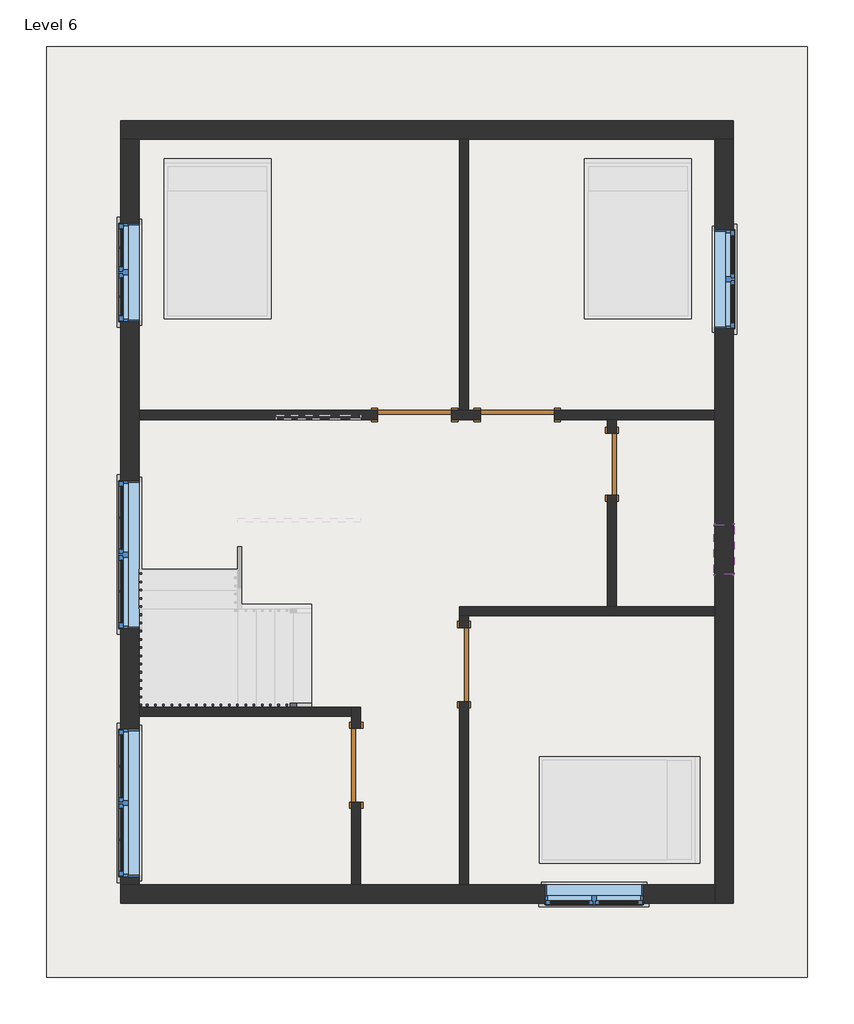
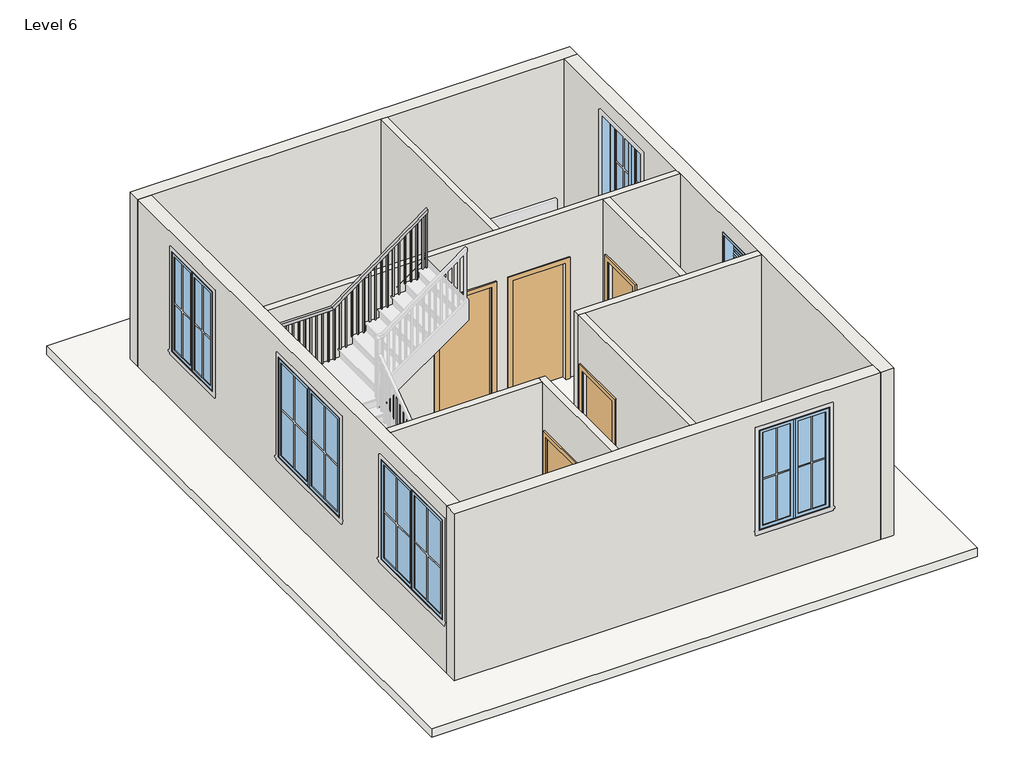
# One storey, part 1 of 2: 11 walls, 6 windows, 5 doors, 1 railing, 1 roof.
"""IFC4 building model written with IfcOpenShell, lengths in millimetres."""

from ifc_helpers import new_model, si_unit, frame, origin, place, context, project, spatial, polyline, outline, extrude, faceted_brep, transform, mapped, element, save
from components import door_f2b275c1, single_flush_door_3_e5f9f3c4, single_flush_door_3_305aa2a5, window_casement_double_win_4_6ca1769e, window_casement_double_win_6_ce442eab, window_f2d8fef0

model = new_model("IFC4")

# Units and contexts
model_context = context("Model", 3, world=origin())
ifc_project = project(units=[si_unit("LENGTHUNIT", "METRE", prefix="MILLI")], contexts=[model_context])

# Site, building, storey
site = spatial("IfcSite", under=ifc_project)
building = spatial("IfcBuilding", under=site)
storey = spatial("IfcBuildingStorey", under=building, Name="Level 6", Elevation=15849.6)

# Doors
placement = place(None, origin())
door_shape = door_f2b275c1(model_context)
element("IfcDoor", 1, ObjectType="Single-Flush : 2'6\"", at=placement, inside=storey, context=model_context, shape_type="MappedRepresentation", body=[
    mapped(door_shape, transform((1031.6394609, 262.5126239, 15849.6), x_axis=(0.0, 1.0, 0.0), y_axis=(-1.0, 0.0, 0.0), z_axis=(0.0, 0.0, 1.0))),
])
single_flush_door_3_shape = single_flush_door_3_e5f9f3c4(model_context)
element("IfcDoor", 2, ObjectType="Single-Flush : door 3'", at=placement, inside=storey, context=model_context, shape_type="MappedRepresentation", body=[
    mapped(single_flush_door_3_shape, transform((-1406.7605391, 872.1126239, 15849.6), x_axis=(1.0, 0.0, 0.0), y_axis=(0.0, 1.0, 0.0), z_axis=(0.0, 0.0, 1.0))),
])
element("IfcDoor", 3, ObjectType="Single-Flush : door 3'", at=placement, inside=storey, context=model_context, shape_type="MappedRepresentation", body=[
    mapped(single_flush_door_3_shape, transform((-2130.6605391, -3458.5873761, 15849.6), x_axis=(0.0, 1.0, 0.0), y_axis=(-1.0, 0.0, 0.0), z_axis=(0.0, 0.0, 1.0))),
])
single_flush_door_3_2_shape = single_flush_door_3_305aa2a5(model_context)
element("IfcDoor", 4, ObjectType="Single-Flush : door 3'", at=placement, inside=storey, context=model_context, shape_type="MappedRepresentation", body=[
    mapped(single_flush_door_3_2_shape, transform((-136.7605391, 872.1126239, 15849.6), x_axis=(-1.0, 0.0, 0.0), y_axis=(0.0, -1.0, 0.0), z_axis=(0.0, 0.0, 1.0))),
])
element("IfcDoor", 5, ObjectType="Single-Flush : door 3'", at=placement, inside=storey, context=model_context, shape_type="MappedRepresentation", body=[
    mapped(single_flush_door_3_2_shape, transform((-797.1605391, -2213.9873761, 15849.6), x_axis=(0.0, 1.0, 0.0), y_axis=(-1.0, 0.0, 0.0), z_axis=(0.0, 0.0, 1.0))),
])

# Railing
element("IfcRailing", 6, ObjectType="Handrail - Rectangular", at=placement, inside=storey, context=model_context, shape_type="SolidModel", body=[
    faceted_brep([(-2683.1105391, -2741.0373761, 16924.4210526), (-2683.1105391, -2741.0373761, 16862.3605986), (-2683.1105391, -2690.2373761, 16862.3605986), (-2683.1105391, -2690.2373761, 16924.4210526), (-3698.24463, -2741.0373761, 17636.7958533), (-3714.290777, -2741.0373761, 17585.9958533), (-3714.290777, -2690.2373761, 17585.9958533), (-3698.24463, -2690.2373761, 17636.7958533), (-4816.7105391, -2741.0373761, 17636.7958533), (-4816.7105391, -2741.0373761, 17585.9958533), (-4765.9105391, -2690.2373761, 17585.9958533), (-4765.9105391, -2690.2373761, 17636.7958533), (-4816.7105391, -1646.8618205, 17636.7958533), (-4816.7105391, -1630.5188912, 17585.9958533), (-4765.9105391, -1630.5188912, 17585.9958533), (-4765.9105391, -1646.8618205, 17636.7958533), (-4816.7105391, -308.3947094, 18597.4181818), (-4816.7105391, -292.0517801, 18546.6181818), (-4765.9105391, -292.0517801, 18546.6181818), (-4765.9105391, -308.3947094, 18597.4181818), (-4816.7105391, 814.9626239, 18597.4181818), (-4816.7105391, 814.9626239, 18546.6181818), (-4765.9105391, 764.1626239, 18546.6181818), (-4765.9105391, 764.1626239, 18597.4181818), (-3721.871578, 814.9626239, 18597.4181818), (-3705.1770744, 814.9626239, 18546.6181818), (-3705.1770744, 764.1626239, 18546.6181818), (-3721.871578, 764.1626239, 18597.4181818), (-2073.5105391, 814.9626239, 19812.0), (-2073.5105391, 764.1626239, 19812.0), (-2073.5105391, 764.1626239, 19748.8987868), (-2073.5105391, 814.9626239, 19748.8987868)], [[[0, 1, 2, 3]], [[1, 0, 4, 5]], [[2, 1, 5, 6]], [[3, 2, 6, 7]], [[0, 3, 7, 4]], [[5, 4, 8, 9]], [[6, 5, 9, 10]], [[7, 6, 10, 11]], [[4, 7, 11, 8]], [[9, 8, 12, 13]], [[10, 9, 13, 14]], [[11, 10, 14, 15]], [[8, 11, 15, 12]], [[13, 12, 16, 17]], [[14, 13, 17, 18]], [[15, 14, 18, 19]], [[12, 15, 19, 16]], [[17, 16, 20, 21]], [[18, 17, 21, 22]], [[19, 18, 22, 23]], [[16, 19, 23, 20]], [[21, 20, 24, 25]], [[22, 21, 25, 26]], [[23, 22, 26, 27]], [[20, 23, 27, 24]], [[28, 29, 30, 31]], [[25, 24, 28, 31]], [[26, 25, 31, 30]], [[27, 26, 30, 29]], [[24, 27, 29, 28]]]),
    extrude(outline(polyline([(19685.7329974, -2159.2355391), (18737.1789474, -2159.2355391), (18737.1789474, -2140.1855391), (19699.7698395, -2140.1855391), (19685.7329974, -2159.2355391)])), frame((0.0, 780.0376239, 0.0), z_axis=(0.0, 1.0, 0.0), x_axis=(0.0, 0.0, 1.0)), (0.0, 0.0, 1.0), 19.05),
    extrude(outline(polyline([(19610.8698395, -2260.8355391), (18576.7578947, -2260.8355391), (18576.7578947, -2241.7855391), (19624.9066816, -2241.7855391), (19610.8698395, -2260.8355391)])), frame((0.0, 780.0376239, 0.0), z_axis=(0.0, 1.0, 0.0), x_axis=(0.0, 0.0, 1.0)), (0.0, 0.0, 1.0), 19.05),
    extrude(outline(polyline([(19536.0066816, -2362.4355391), (18576.7578947, -2362.4355391), (18576.7578947, -2343.3855391), (19550.0435237, -2343.3855391), (19536.0066816, -2362.4355391)])), frame((0.0, 780.0376239, 0.0), z_axis=(0.0, 1.0, 0.0), x_axis=(0.0, 0.0, 1.0)), (0.0, 0.0, 1.0), 19.05),
    extrude(outline(polyline([(19461.1435237, -2464.0355391), (18576.7578947, -2464.0355391), (18576.7578947, -2444.9855391), (19475.1803658, -2444.9855391), (19461.1435237, -2464.0355391)])), frame((0.0, 780.0376239, 0.0), z_axis=(0.0, 1.0, 0.0), x_axis=(0.0, 0.0, 1.0)), (0.0, 0.0, 1.0), 19.05),
    extrude(outline(polyline([(19386.2803658, -2565.6355391), (18416.3368421, -2565.6355391), (18416.3368421, -2546.5855391), (19400.3172079, -2546.5855391), (19386.2803658, -2565.6355391)])), frame((0.0, 780.0376239, 0.0), z_axis=(0.0, 1.0, 0.0), x_axis=(0.0, 0.0, 1.0)), (0.0, 0.0, 1.0), 19.05),
    extrude(outline(polyline([(19311.4172079, -2667.2355391), (18416.3368421, -2667.2355391), (18416.3368421, -2648.1855391), (19325.45405, -2648.1855391), (19311.4172079, -2667.2355391)])), frame((0.0, 780.0376239, 0.0), z_axis=(0.0, 1.0, 0.0), x_axis=(0.0, 0.0, 1.0)), (0.0, 0.0, 1.0), 19.05),
    extrude(outline(polyline([(19236.55405, -2768.8355391), (18255.9157895, -2768.8355391), (18255.9157895, -2749.7855391), (19250.5908921, -2749.7855391), (19236.55405, -2768.8355391)])), frame((0.0, 780.0376239, 0.0), z_axis=(0.0, 1.0, 0.0), x_axis=(0.0, 0.0, 1.0)), (0.0, 0.0, 1.0), 19.05),
    extrude(outline(polyline([(19161.6908921, -2870.4355391), (18255.9157895, -2870.4355391), (18255.9157895, -2851.3855391), (19175.7277342, -2851.3855391), (19161.6908921, -2870.4355391)])), frame((0.0, 780.0376239, 0.0), z_axis=(0.0, 1.0, 0.0), x_axis=(0.0, 0.0, 1.0)), (0.0, 0.0, 1.0), 19.05),
    extrude(outline(polyline([(19086.8277342, -2972.0355391), (18095.4947368, -2972.0355391), (18095.4947368, -2952.9855391), (19100.8645763, -2952.9855391), (19086.8277342, -2972.0355391)])), frame((0.0, 780.0376239, 0.0), z_axis=(0.0, 1.0, 0.0), x_axis=(0.0, 0.0, 1.0)), (0.0, 0.0, 1.0), 19.05),
    extrude(outline(polyline([(19011.9645763, -3073.6355391), (18095.4947368, -3073.6355391), (18095.4947368, -3054.5855391), (19026.0014184, -3054.5855391), (19011.9645763, -3073.6355391)])), frame((0.0, 780.0376239, 0.0), z_axis=(0.0, 1.0, 0.0), x_axis=(0.0, 0.0, 1.0)), (0.0, 0.0, 1.0), 19.05),
    extrude(outline(polyline([(18937.1014184, -3175.2355391), (17935.0736842, -3175.2355391), (17935.0736842, -3156.1855391), (18951.1382605, -3156.1855391), (18937.1014184, -3175.2355391)])), frame((0.0, 780.0376239, 0.0), z_axis=(0.0, 1.0, 0.0), x_axis=(0.0, 0.0, 1.0)), (0.0, 0.0, 1.0), 19.05),
    extrude(outline(polyline([(18862.2382605, -3276.8355391), (17935.0736842, -3276.8355391), (17935.0736842, -3257.7855391), (18876.2751026, -3257.7855391), (18862.2382605, -3276.8355391)])), frame((0.0, 780.0376239, 0.0), z_axis=(0.0, 1.0, 0.0), x_axis=(0.0, 0.0, 1.0)), (0.0, 0.0, 1.0), 19.05),
    extrude(outline(polyline([(18787.3751026, -3378.4355391), (17935.0736842, -3378.4355391), (17935.0736842, -3359.3855391), (18801.4119447, -3359.3855391), (18787.3751026, -3378.4355391)])), frame((0.0, 780.0376239, 0.0), z_axis=(0.0, 1.0, 0.0), x_axis=(0.0, 0.0, 1.0)), (0.0, 0.0, 1.0), 19.05),
    extrude(outline(polyline([(18712.5119447, -3480.0355391), (17774.6526316, -3480.0355391), (17774.6526316, -3460.9855391), (18726.5487868, -3460.9855391), (18712.5119447, -3480.0355391)])), frame((0.0, 780.0376239, 0.0), z_axis=(0.0, 1.0, 0.0), x_axis=(0.0, 0.0, 1.0)), (0.0, 0.0, 1.0), 19.05),
    extrude(outline(polyline([(18637.6487868, -3581.6355391), (17774.6526316, -3581.6355391), (17774.6526316, -3562.5855391), (18651.6856289, -3562.5855391), (18637.6487868, -3581.6355391)])), frame((0.0, 780.0376239, 0.0), z_axis=(0.0, 1.0, 0.0), x_axis=(0.0, 0.0, 1.0)), (0.0, 0.0, 1.0), 19.05),
    extrude(outline(polyline([(18562.7856289, -3683.2355391), (17614.2315789, -3683.2355391), (17614.2315789, -3664.1855391), (18576.822471, -3664.1855391), (18562.7856289, -3683.2355391)])), frame((0.0, 780.0376239, 0.0), z_axis=(0.0, 1.0, 0.0), x_axis=(0.0, 0.0, 1.0)), (0.0, 0.0, 1.0), 19.05),
    extrude(outline(polyline([(-3784.8355391, 799.0876239), (-3765.7855391, 799.0876239), (-3765.7855391, 780.0376239), (-3784.8355391, 780.0376239), (-3784.8355391, 799.0876239)])), frame((0.0, 0.0, 17614.2315789), z_axis=(0.0, 0.0, 1.0), x_axis=(1.0, 0.0, 0.0)), (0.0, 0.0, 1.0), 932.3866029),
    extrude(outline(polyline([(-3886.4355391, 799.0876239), (-3867.3855391, 799.0876239), (-3867.3855391, 780.0376239), (-3886.4355391, 780.0376239), (-3886.4355391, 799.0876239)])), frame((0.0, 0.0, 17614.2315789), z_axis=(0.0, 0.0, 1.0), x_axis=(1.0, 0.0, 0.0)), (0.0, 0.0, 1.0), 932.3866029),
    extrude(outline(polyline([(-3988.0355391, 799.0876239), (-3968.9855391, 799.0876239), (-3968.9855391, 780.0376239), (-3988.0355391, 780.0376239), (-3988.0355391, 799.0876239)])), frame((0.0, 0.0, 17614.2315789), z_axis=(0.0, 0.0, 1.0), x_axis=(1.0, 0.0, 0.0)), (0.0, 0.0, 1.0), 932.3866029),
    extrude(outline(polyline([(-4089.6355391, 799.0876239), (-4070.5855391, 799.0876239), (-4070.5855391, 780.0376239), (-4089.6355391, 780.0376239), (-4089.6355391, 799.0876239)])), frame((0.0, 0.0, 17614.2315789), z_axis=(0.0, 0.0, 1.0), x_axis=(1.0, 0.0, 0.0)), (0.0, 0.0, 1.0), 932.3866029),
    extrude(outline(polyline([(-4191.2355391, 799.0876239), (-4172.1855391, 799.0876239), (-4172.1855391, 780.0376239), (-4191.2355391, 780.0376239), (-4191.2355391, 799.0876239)])), frame((0.0, 0.0, 17614.2315789), z_axis=(0.0, 0.0, 1.0), x_axis=(1.0, 0.0, 0.0)), (0.0, 0.0, 1.0), 932.3866029),
    extrude(outline(polyline([(-4292.8355391, 799.0876239), (-4273.7855391, 799.0876239), (-4273.7855391, 780.0376239), (-4292.8355391, 780.0376239), (-4292.8355391, 799.0876239)])), frame((0.0, 0.0, 17614.2315789), z_axis=(0.0, 0.0, 1.0), x_axis=(1.0, 0.0, 0.0)), (0.0, 0.0, 1.0), 932.3866029),
    extrude(outline(polyline([(-4394.4355391, 799.0876239), (-4375.3855391, 799.0876239), (-4375.3855391, 780.0376239), (-4394.4355391, 780.0376239), (-4394.4355391, 799.0876239)])), frame((0.0, 0.0, 17614.2315789), z_axis=(0.0, 0.0, 1.0), x_axis=(1.0, 0.0, 0.0)), (0.0, 0.0, 1.0), 932.3866029),
    extrude(outline(polyline([(-4496.0355391, 799.0876239), (-4476.9855391, 799.0876239), (-4476.9855391, 780.0376239), (-4496.0355391, 780.0376239), (-4496.0355391, 799.0876239)])), frame((0.0, 0.0, 17614.2315789), z_axis=(0.0, 0.0, 1.0), x_axis=(1.0, 0.0, 0.0)), (0.0, 0.0, 1.0), 932.3866029),
    extrude(outline(polyline([(-4597.6355391, 799.0876239), (-4578.5855391, 799.0876239), (-4578.5855391, 780.0376239), (-4597.6355391, 780.0376239), (-4597.6355391, 799.0876239)])), frame((0.0, 0.0, 17614.2315789), z_axis=(0.0, 0.0, 1.0), x_axis=(1.0, 0.0, 0.0)), (0.0, 0.0, 1.0), 932.3866029),
    extrude(outline(polyline([(-4699.2355391, 799.0876239), (-4680.1855391, 799.0876239), (-4680.1855391, 780.0376239), (-4699.2355391, 780.0376239), (-4699.2355391, 799.0876239)])), frame((0.0, 0.0, 17614.2315789), z_axis=(0.0, 0.0, 1.0), x_axis=(1.0, 0.0, 0.0)), (0.0, 0.0, 1.0), 932.3866029),
    extrude(outline(polyline([(-4800.8355391, 729.2376239), (-4800.8355391, 748.2876239), (-4781.7855391, 748.2876239), (-4781.7855391, 729.2376239), (-4800.8355391, 729.2376239)])), frame((0.0, 0.0, 17614.2315789), z_axis=(0.0, 0.0, 1.0), x_axis=(1.0, 0.0, 0.0)), (0.0, 0.0, 1.0), 932.3866029),
    extrude(outline(polyline([(-4800.8355391, 627.6376239), (-4800.8355391, 646.6876239), (-4781.7855391, 646.6876239), (-4781.7855391, 627.6376239), (-4800.8355391, 627.6376239)])), frame((0.0, 0.0, 17614.2315789), z_axis=(0.0, 0.0, 1.0), x_axis=(1.0, 0.0, 0.0)), (0.0, 0.0, 1.0), 932.3866029),
    extrude(outline(polyline([(-4800.8355391, 526.0376239), (-4800.8355391, 545.0876239), (-4781.7855391, 545.0876239), (-4781.7855391, 526.0376239), (-4800.8355391, 526.0376239)])), frame((0.0, 0.0, 17614.2315789), z_axis=(0.0, 0.0, 1.0), x_axis=(1.0, 0.0, 0.0)), (0.0, 0.0, 1.0), 932.3866029),
    extrude(outline(polyline([(-4800.8355391, 424.4376239), (-4800.8355391, 443.4876239), (-4781.7855391, 443.4876239), (-4781.7855391, 424.4376239), (-4800.8355391, 424.4376239)])), frame((0.0, 0.0, 17614.2315789), z_axis=(0.0, 0.0, 1.0), x_axis=(1.0, 0.0, 0.0)), (0.0, 0.0, 1.0), 932.3866029),
    extrude(outline(polyline([(-4800.8355391, 322.8376239), (-4800.8355391, 341.8876239), (-4781.7855391, 341.8876239), (-4781.7855391, 322.8376239), (-4800.8355391, 322.8376239)])), frame((0.0, 0.0, 17614.2315789), z_axis=(0.0, 0.0, 1.0), x_axis=(1.0, 0.0, 0.0)), (0.0, 0.0, 1.0), 932.3866029),
    extrude(outline(polyline([(-4800.8355391, 221.2376239), (-4800.8355391, 240.2876239), (-4781.7855391, 240.2876239), (-4781.7855391, 221.2376239), (-4800.8355391, 221.2376239)])), frame((0.0, 0.0, 17614.2315789), z_axis=(0.0, 0.0, 1.0), x_axis=(1.0, 0.0, 0.0)), (0.0, 0.0, 1.0), 932.3866029),
    extrude(outline(polyline([(-4800.8355391, 119.6376239), (-4800.8355391, 138.6876239), (-4781.7855391, 138.6876239), (-4781.7855391, 119.6376239), (-4800.8355391, 119.6376239)])), frame((0.0, 0.0, 17614.2315789), z_axis=(0.0, 0.0, 1.0), x_axis=(1.0, 0.0, 0.0)), (0.0, 0.0, 1.0), 932.3866029),
    extrude(outline(polyline([(-4800.8355391, 18.0376239), (-4800.8355391, 37.0876239), (-4781.7855391, 37.0876239), (-4781.7855391, 18.0376239), (-4800.8355391, 18.0376239)])), frame((0.0, 0.0, 17614.2315789), z_axis=(0.0, 0.0, 1.0), x_axis=(1.0, 0.0, 0.0)), (0.0, 0.0, 1.0), 932.3866029),
    extrude(outline(polyline([(-4800.8355391, -83.5623761), (-4800.8355391, -64.5123761), (-4781.7855391, -64.5123761), (-4781.7855391, -83.5623761), (-4800.8355391, -83.5623761)])), frame((0.0, 0.0, 17614.2315789), z_axis=(0.0, 0.0, 1.0), x_axis=(1.0, 0.0, 0.0)), (0.0, 0.0, 1.0), 932.3866029),
    extrude(outline(polyline([(-4800.8355391, -185.1623761), (-4800.8355391, -166.1123761), (-4781.7855391, -166.1123761), (-4781.7855391, -185.1623761), (-4800.8355391, -185.1623761)])), frame((0.0, 0.0, 17614.2315789), z_axis=(0.0, 0.0, 1.0), x_axis=(1.0, 0.0, 0.0)), (0.0, 0.0, 1.0), 932.3866029),
    extrude(outline(polyline([(-4800.8355391, -286.7623761), (-4800.8355391, -267.7123761), (-4781.7855391, -267.7123761), (-4781.7855391, -286.7623761), (-4800.8355391, -286.7623761)])), frame((0.0, 0.0, 17614.2315789), z_axis=(0.0, 0.0, 1.0), x_axis=(1.0, 0.0, 0.0)), (0.0, 0.0, 1.0), 932.3866029),
    extrude(outline(polyline([(-369.3123761, 18491.1679933), (-369.3123761, 17614.2315789), (-388.3623761, 17614.2315789), (-388.3623761, 18477.4957445), (-369.3123761, 18491.1679933)])), frame((-4800.8355391, 0.0, 0.0), z_axis=(1.0, 0.0, 0.0), x_axis=(0.0, 1.0, 0.0)), (0.0, 0.0, 1.0), 19.05),
    extrude(outline(polyline([(-470.9123761, 18418.249333), (-470.9123761, 17453.8105263), (-489.9623761, 17453.8105263), (-489.9623761, 18404.5770842), (-470.9123761, 18418.249333)])), frame((-4800.8355391, 0.0, 0.0), z_axis=(1.0, 0.0, 0.0), x_axis=(0.0, 1.0, 0.0)), (0.0, 0.0, 1.0), 19.05),
    extrude(outline(polyline([(-572.5123761, 18345.3306727), (-572.5123761, 17453.8105263), (-591.5623761, 17453.8105263), (-591.5623761, 18331.6584239), (-572.5123761, 18345.3306727)])), frame((-4800.8355391, 0.0, 0.0), z_axis=(1.0, 0.0, 0.0), x_axis=(0.0, 1.0, 0.0)), (0.0, 0.0, 1.0), 19.05),
    extrude(outline(polyline([(-674.1123761, 18272.4120124), (-674.1123761, 17293.3894737), (-693.1623761, 17293.3894737), (-693.1623761, 18258.7397636), (-674.1123761, 18272.4120124)])), frame((-4800.8355391, 0.0, 0.0), z_axis=(1.0, 0.0, 0.0), x_axis=(0.0, 1.0, 0.0)), (0.0, 0.0, 1.0), 19.05),
    extrude(outline(polyline([(-775.7123761, 18199.4933521), (-775.7123761, 17293.3894737), (-794.7623761, 17293.3894737), (-794.7623761, 18185.8211033), (-775.7123761, 18199.4933521)])), frame((-4800.8355391, 0.0, 0.0), z_axis=(1.0, 0.0, 0.0), x_axis=(0.0, 1.0, 0.0)), (0.0, 0.0, 1.0), 19.05),
    extrude(outline(polyline([(-877.3123761, 18126.5746919), (-877.3123761, 17132.9684211), (-896.3623761, 17132.9684211), (-896.3623761, 18112.902443), (-877.3123761, 18126.5746919)])), frame((-4800.8355391, 0.0, 0.0), z_axis=(1.0, 0.0, 0.0), x_axis=(0.0, 1.0, 0.0)), (0.0, 0.0, 1.0), 19.05),
    extrude(outline(polyline([(-978.9123761, 18053.6560316), (-978.9123761, 17132.9684211), (-997.9623761, 17132.9684211), (-997.9623761, 18039.9837828), (-978.9123761, 18053.6560316)])), frame((-4800.8355391, 0.0, 0.0), z_axis=(1.0, 0.0, 0.0), x_axis=(0.0, 1.0, 0.0)), (0.0, 0.0, 1.0), 19.05),
    extrude(outline(polyline([(-1080.5123761, 17980.7373713), (-1080.5123761, 16972.5473684), (-1099.5623761, 16972.5473684), (-1099.5623761, 17967.0651225), (-1080.5123761, 17980.7373713)])), frame((-4800.8355391, 0.0, 0.0), z_axis=(1.0, 0.0, 0.0), x_axis=(0.0, 1.0, 0.0)), (0.0, 0.0, 1.0), 19.05),
    extrude(outline(polyline([(-1182.1123761, 17907.818711), (-1182.1123761, 16972.5473684), (-1201.1623761, 16972.5473684), (-1201.1623761, 17894.1464622), (-1182.1123761, 17907.818711)])), frame((-4800.8355391, 0.0, 0.0), z_axis=(1.0, 0.0, 0.0), x_axis=(0.0, 1.0, 0.0)), (0.0, 0.0, 1.0), 19.05),
    extrude(outline(polyline([(-1283.7123761, 17834.9000507), (-1283.7123761, 16972.5473684), (-1302.7623761, 16972.5473684), (-1302.7623761, 17821.2278019), (-1283.7123761, 17834.9000507)])), frame((-4800.8355391, 0.0, 0.0), z_axis=(1.0, 0.0, 0.0), x_axis=(0.0, 1.0, 0.0)), (0.0, 0.0, 1.0), 19.05),
    extrude(outline(polyline([(-1385.3123761, 17761.9813904), (-1385.3123761, 16812.1263158), (-1404.3623761, 16812.1263158), (-1404.3623761, 17748.3091416), (-1385.3123761, 17761.9813904)])), frame((-4800.8355391, 0.0, 0.0), z_axis=(1.0, 0.0, 0.0), x_axis=(0.0, 1.0, 0.0)), (0.0, 0.0, 1.0), 19.05),
    extrude(outline(polyline([(-1486.9123761, 17689.0627301), (-1486.9123761, 16812.1263158), (-1505.9623761, 16812.1263158), (-1505.9623761, 17675.3904813), (-1486.9123761, 17689.0627301)])), frame((-4800.8355391, 0.0, 0.0), z_axis=(1.0, 0.0, 0.0), x_axis=(0.0, 1.0, 0.0)), (0.0, 0.0, 1.0), 19.05),
    extrude(outline(polyline([(-1588.5123761, 17616.1440698), (-1588.5123761, 16651.7052632), (-1607.5623761, 16651.7052632), (-1607.5623761, 17602.471821), (-1588.5123761, 17616.1440698)])), frame((-4800.8355391, 0.0, 0.0), z_axis=(1.0, 0.0, 0.0), x_axis=(0.0, 1.0, 0.0)), (0.0, 0.0, 1.0), 19.05),
    extrude(outline(polyline([(-4800.8355391, -1709.1623761), (-4800.8355391, -1690.1123761), (-4781.7855391, -1690.1123761), (-4781.7855391, -1709.1623761), (-4800.8355391, -1709.1623761)])), frame((0.0, 0.0, 16651.7052632), z_axis=(0.0, 0.0, 1.0), x_axis=(1.0, 0.0, 0.0)), (0.0, 0.0, 1.0), 934.2905901),
    extrude(outline(polyline([(-4800.8355391, -1810.7623761), (-4800.8355391, -1791.7123761), (-4781.7855391, -1791.7123761), (-4781.7855391, -1810.7623761), (-4800.8355391, -1810.7623761)])), frame((0.0, 0.0, 16651.7052632), z_axis=(0.0, 0.0, 1.0), x_axis=(1.0, 0.0, 0.0)), (0.0, 0.0, 1.0), 934.2905901),
    extrude(outline(polyline([(-4800.8355391, -1912.3623761), (-4800.8355391, -1893.3123761), (-4781.7855391, -1893.3123761), (-4781.7855391, -1912.3623761), (-4800.8355391, -1912.3623761)])), frame((0.0, 0.0, 16651.7052632), z_axis=(0.0, 0.0, 1.0), x_axis=(1.0, 0.0, 0.0)), (0.0, 0.0, 1.0), 934.2905901),
    extrude(outline(polyline([(-4800.8355391, -2013.9623761), (-4800.8355391, -1994.9123761), (-4781.7855391, -1994.9123761), (-4781.7855391, -2013.9623761), (-4800.8355391, -2013.9623761)])), frame((0.0, 0.0, 16651.7052632), z_axis=(0.0, 0.0, 1.0), x_axis=(1.0, 0.0, 0.0)), (0.0, 0.0, 1.0), 934.2905901),
    extrude(outline(polyline([(-4800.8355391, -2115.5623761), (-4800.8355391, -2096.5123761), (-4781.7855391, -2096.5123761), (-4781.7855391, -2115.5623761), (-4800.8355391, -2115.5623761)])), frame((0.0, 0.0, 16651.7052632), z_axis=(0.0, 0.0, 1.0), x_axis=(1.0, 0.0, 0.0)), (0.0, 0.0, 1.0), 934.2905901),
    extrude(outline(polyline([(-4800.8355391, -2217.1623761), (-4800.8355391, -2198.1123761), (-4781.7855391, -2198.1123761), (-4781.7855391, -2217.1623761), (-4800.8355391, -2217.1623761)])), frame((0.0, 0.0, 16651.7052632), z_axis=(0.0, 0.0, 1.0), x_axis=(1.0, 0.0, 0.0)), (0.0, 0.0, 1.0), 934.2905901),
    extrude(outline(polyline([(-4800.8355391, -2318.7623761), (-4800.8355391, -2299.7123761), (-4781.7855391, -2299.7123761), (-4781.7855391, -2318.7623761), (-4800.8355391, -2318.7623761)])), frame((0.0, 0.0, 16651.7052632), z_axis=(0.0, 0.0, 1.0), x_axis=(1.0, 0.0, 0.0)), (0.0, 0.0, 1.0), 934.2905901),
    extrude(outline(polyline([(-4800.8355391, -2420.3623761), (-4800.8355391, -2401.3123761), (-4781.7855391, -2401.3123761), (-4781.7855391, -2420.3623761), (-4800.8355391, -2420.3623761)])), frame((0.0, 0.0, 16651.7052632), z_axis=(0.0, 0.0, 1.0), x_axis=(1.0, 0.0, 0.0)), (0.0, 0.0, 1.0), 934.2905901),
    extrude(outline(polyline([(-4800.8355391, -2521.9623761), (-4800.8355391, -2502.9123761), (-4781.7855391, -2502.9123761), (-4781.7855391, -2521.9623761), (-4800.8355391, -2521.9623761)])), frame((0.0, 0.0, 16651.7052632), z_axis=(0.0, 0.0, 1.0), x_axis=(1.0, 0.0, 0.0)), (0.0, 0.0, 1.0), 934.2905901),
    extrude(outline(polyline([(-4800.8355391, -2623.5623761), (-4800.8355391, -2604.5123761), (-4781.7855391, -2604.5123761), (-4781.7855391, -2623.5623761), (-4800.8355391, -2623.5623761)])), frame((0.0, 0.0, 16651.7052632), z_axis=(0.0, 0.0, 1.0), x_axis=(1.0, 0.0, 0.0)), (0.0, 0.0, 1.0), 934.2905901),
    extrude(outline(polyline([(-4705.5855391, -2725.1623761), (-4724.6355391, -2725.1623761), (-4724.6355391, -2706.1123761), (-4705.5855391, -2706.1123761), (-4705.5855391, -2725.1623761)])), frame((0.0, 0.0, 16651.7052632), z_axis=(0.0, 0.0, 1.0), x_axis=(1.0, 0.0, 0.0)), (0.0, 0.0, 1.0), 934.2905901),
    extrude(outline(polyline([(-4603.9855391, -2725.1623761), (-4623.0355391, -2725.1623761), (-4623.0355391, -2706.1123761), (-4603.9855391, -2706.1123761), (-4603.9855391, -2725.1623761)])), frame((0.0, 0.0, 16651.7052632), z_axis=(0.0, 0.0, 1.0), x_axis=(1.0, 0.0, 0.0)), (0.0, 0.0, 1.0), 934.2905901),
    extrude(outline(polyline([(-4502.3855391, -2725.1623761), (-4521.4355391, -2725.1623761), (-4521.4355391, -2706.1123761), (-4502.3855391, -2706.1123761), (-4502.3855391, -2725.1623761)])), frame((0.0, 0.0, 16651.7052632), z_axis=(0.0, 0.0, 1.0), x_axis=(1.0, 0.0, 0.0)), (0.0, 0.0, 1.0), 934.2905901),
    extrude(outline(polyline([(-4400.7855391, -2725.1623761), (-4419.8355391, -2725.1623761), (-4419.8355391, -2706.1123761), (-4400.7855391, -2706.1123761), (-4400.7855391, -2725.1623761)])), frame((0.0, 0.0, 16651.7052632), z_axis=(0.0, 0.0, 1.0), x_axis=(1.0, 0.0, 0.0)), (0.0, 0.0, 1.0), 934.2905901),
    extrude(outline(polyline([(-4299.1855391, -2725.1623761), (-4318.2355391, -2725.1623761), (-4318.2355391, -2706.1123761), (-4299.1855391, -2706.1123761), (-4299.1855391, -2725.1623761)])), frame((0.0, 0.0, 16651.7052632), z_axis=(0.0, 0.0, 1.0), x_axis=(1.0, 0.0, 0.0)), (0.0, 0.0, 1.0), 934.2905901),
    extrude(outline(polyline([(-4197.5855391, -2725.1623761), (-4216.6355391, -2725.1623761), (-4216.6355391, -2706.1123761), (-4197.5855391, -2706.1123761), (-4197.5855391, -2725.1623761)])), frame((0.0, 0.0, 16651.7052632), z_axis=(0.0, 0.0, 1.0), x_axis=(1.0, 0.0, 0.0)), (0.0, 0.0, 1.0), 934.2905901),
    extrude(outline(polyline([(-4095.9855391, -2725.1623761), (-4115.0355391, -2725.1623761), (-4115.0355391, -2706.1123761), (-4095.9855391, -2706.1123761), (-4095.9855391, -2725.1623761)])), frame((0.0, 0.0, 16651.7052632), z_axis=(0.0, 0.0, 1.0), x_axis=(1.0, 0.0, 0.0)), (0.0, 0.0, 1.0), 934.2905901),
    extrude(outline(polyline([(-3994.3855391, -2725.1623761), (-4013.4355391, -2725.1623761), (-4013.4355391, -2706.1123761), (-3994.3855391, -2706.1123761), (-3994.3855391, -2725.1623761)])), frame((0.0, 0.0, 16651.7052632), z_axis=(0.0, 0.0, 1.0), x_axis=(1.0, 0.0, 0.0)), (0.0, 0.0, 1.0), 934.2905901),
    extrude(outline(polyline([(-3892.7855391, -2725.1623761), (-3911.8355391, -2725.1623761), (-3911.8355391, -2706.1123761), (-3892.7855391, -2706.1123761), (-3892.7855391, -2725.1623761)])), frame((0.0, 0.0, 16651.7052632), z_axis=(0.0, 0.0, 1.0), x_axis=(1.0, 0.0, 0.0)), (0.0, 0.0, 1.0), 934.2905901),
    extrude(outline(polyline([(-3791.1855391, -2725.1623761), (-3810.2355391, -2725.1623761), (-3810.2355391, -2706.1123761), (-3791.1855391, -2706.1123761), (-3791.1855391, -2725.1623761)])), frame((0.0, 0.0, 16651.7052632), z_axis=(0.0, 0.0, 1.0), x_axis=(1.0, 0.0, 0.0)), (0.0, 0.0, 1.0), 934.2905901),
    extrude(outline(polyline([(-3689.5855391, -2725.1623761), (-3708.6355391, -2725.1623761), (-3708.6355391, -2706.1123761), (-3689.5855391, -2706.1123761), (-3689.5855391, -2725.1623761)])), frame((0.0, 0.0, 16651.7052632), z_axis=(0.0, 0.0, 1.0), x_axis=(1.0, 0.0, 0.0)), (0.0, 0.0, 1.0), 934.2905901),
    extrude(outline(polyline([(17510.7290196, -3607.0355391), (16651.7052632, -3607.0355391), (16651.7052632, -3587.9855391), (17497.3605986, -3587.9855391), (17510.7290196, -3607.0355391)])), frame((0.0, -2725.1623761, 0.0), z_axis=(0.0, 1.0, 0.0), x_axis=(0.0, 0.0, 1.0)), (0.0, 0.0, 1.0), 19.05),
    extrude(outline(polyline([(17439.430774, -3505.4355391), (16491.2842105, -3505.4355391), (16491.2842105, -3486.3855391), (17426.062353, -3486.3855391), (17439.430774, -3505.4355391)])), frame((0.0, -2725.1623761, 0.0), z_axis=(0.0, 1.0, 0.0), x_axis=(0.0, 0.0, 1.0)), (0.0, 0.0, 1.0), 19.05),
    extrude(outline(polyline([(17368.1325284, -3403.8355391), (16491.2842105, -3403.8355391), (16491.2842105, -3384.7855391), (17354.7641074, -3384.7855391), (17368.1325284, -3403.8355391)])), frame((0.0, -2725.1623761, 0.0), z_axis=(0.0, 1.0, 0.0), x_axis=(0.0, 0.0, 1.0)), (0.0, 0.0, 1.0), 19.05),
    extrude(outline(polyline([(17296.8342828, -3302.2355391), (16330.8631579, -3302.2355391), (16330.8631579, -3283.1855391), (17283.4658617, -3283.1855391), (17296.8342828, -3302.2355391)])), frame((0.0, -2725.1623761, 0.0), z_axis=(0.0, 1.0, 0.0), x_axis=(0.0, 0.0, 1.0)), (0.0, 0.0, 1.0), 19.05),
    extrude(outline(polyline([(17225.5360372, -3200.6355391), (16330.8631579, -3200.6355391), (16330.8631579, -3181.5855391), (17212.1676161, -3181.5855391), (17225.5360372, -3200.6355391)])), frame((0.0, -2725.1623761, 0.0), z_axis=(0.0, 1.0, 0.0), x_axis=(0.0, 0.0, 1.0)), (0.0, 0.0, 1.0), 19.05),
    extrude(outline(polyline([(17154.2377916, -3099.0355391), (16170.4421053, -3099.0355391), (16170.4421053, -3079.9855391), (17140.8693705, -3079.9855391), (17154.2377916, -3099.0355391)])), frame((0.0, -2725.1623761, 0.0), z_axis=(0.0, 1.0, 0.0), x_axis=(0.0, 0.0, 1.0)), (0.0, 0.0, 1.0), 19.05),
    extrude(outline(polyline([(17082.9395459, -2997.4355391), (16170.4421053, -2997.4355391), (16170.4421053, -2978.3855391), (17069.5711249, -2978.3855391), (17082.9395459, -2997.4355391)])), frame((0.0, -2725.1623761, 0.0), z_axis=(0.0, 1.0, 0.0), x_axis=(0.0, 0.0, 1.0)), (0.0, 0.0, 1.0), 19.05),
    extrude(outline(polyline([(17011.6413003, -2895.8355391), (16010.0210526, -2895.8355391), (16010.0210526, -2876.7855391), (16998.2728793, -2876.7855391), (17011.6413003, -2895.8355391)])), frame((0.0, -2725.1623761, 0.0), z_axis=(0.0, 1.0, 0.0), x_axis=(0.0, 0.0, 1.0)), (0.0, 0.0, 1.0), 19.05),
    extrude(outline(polyline([(16940.3430547, -2794.2355391), (16010.0210526, -2794.2355391), (16010.0210526, -2775.1855391), (16926.9746337, -2775.1855391), (16940.3430547, -2794.2355391)])), frame((0.0, -2725.1623761, 0.0), z_axis=(0.0, 1.0, 0.0), x_axis=(0.0, 0.0, 1.0)), (0.0, 0.0, 1.0), 19.05),
    extrude(outline(polyline([(-4800.8355391, 780.0376239), (-4800.8355391, 799.0876239), (-4781.7855391, 799.0876239), (-4781.7855391, 780.0376239), (-4800.8355391, 780.0376239)])), frame((0.0, 0.0, 17614.2315789), z_axis=(0.0, 0.0, 1.0), x_axis=(1.0, 0.0, 0.0)), (0.0, 0.0, 1.0), 932.3866029),
    extrude(outline(polyline([(-4781.7855391, -2725.1623761), (-4800.8355391, -2725.1623761), (-4800.8355391, -2706.1123761), (-4781.7855391, -2706.1123761), (-4781.7855391, -2725.1623761)])), frame((0.0, 0.0, 16651.7052632), z_axis=(0.0, 0.0, 1.0), x_axis=(1.0, 0.0, 0.0)), (0.0, 0.0, 1.0), 934.2905901),
    extrude(outline(polyline([(19734.8619447, -2092.5605391), (18737.1789474, -2092.5605391), (18737.1789474, -2073.5105391), (19748.8987868, -2073.5105391), (19734.8619447, -2092.5605391)])), frame((0.0, 780.0376239, 0.0), z_axis=(0.0, 1.0, 0.0), x_axis=(0.0, 0.0, 1.0)), (0.0, 0.0, 1.0), 19.05),
    extrude(outline(polyline([(16875.7290196, -2702.1605391), (16010.0210526, -2702.1605391), (16010.0210526, -2683.1105391), (16862.3605986, -2683.1105391), (16875.7290196, -2702.1605391)])), frame((0.0, -2725.1623761, 0.0), z_axis=(0.0, 1.0, 0.0), x_axis=(0.0, 0.0, 1.0)), (0.0, 0.0, 1.0), 19.05),
])

# Roof
element("IfcRoof", 7, ObjectType="Generic - 12\"", at=placement, inside=storey, context=model_context, shape_type="SweptSolid", body=[
    extrude(outline(polyline([(-5959.7105391, 5425.0626239), (3450.9894609, 5425.0626239), (3450.9894609, -6081.1373761), (-5959.7105391, -6081.1373761), (-5959.7105391, 5425.0626239)])), frame((0.0, 0.0, 15697.2), z_axis=(0.0, 0.0, 1.0), x_axis=(1.0, 0.0, 0.0)), (0.0, 0.0, 1.0), 152.4),
])

# Walls
element("IfcWall", 8, ObjectType="WALL 4.5\"", at=placement, inside=storey, context=model_context, shape_type="SweptSolid", body=[
    extrude(outline(polyline([(-854.3105391, 929.2626239), (-854.3105391, 4282.0626239), (-740.0105391, 4282.0626239), (-740.0105391, 929.2626239), (-854.3105391, 929.2626239)])), frame((0.0, 0.0, 15849.6), z_axis=(0.0, 0.0, 1.0), x_axis=(1.0, 0.0, 0.0)), (0.0, 0.0, 1.0), 3048.0),
])
element("IfcWall", 9, ObjectType="WALL 4.5\"", at=placement, inside=storey, context=model_context, shape_type="Brep", body=[
    faceted_brep([(-949.5605391, 814.9626239, 15849.6), (-593.9605391, 814.9626239, 15849.6), (-593.9605391, 814.9626239, 17983.2), (320.4394609, 814.9626239, 17983.2), (320.4394609, 814.9626239, 15849.6), (974.4894609, 814.9626239, 15849.6), (1088.7894609, 814.9626239, 15849.6), (2307.9894609, 814.9626239, 15849.6), (2307.9894609, 814.9626239, 18897.6), (1088.7894609, 814.9626239, 18897.6), (974.4894609, 814.9626239, 18897.6), (-4816.7105391, 814.9626239, 18897.6), (-4816.7105391, 814.9626239, 15849.6), (-1863.9605391, 814.9626239, 15849.6), (-1863.9605391, 814.9626239, 17983.2), (-949.5605391, 814.9626239, 17983.2), (-593.9605391, 929.2626239, 17983.2), (-593.9605391, 929.2626239, 15849.6), (-740.0105391, 929.2626239, 15849.6), (-854.3105391, 929.2626239, 15849.6), (-949.5605391, 929.2626239, 15849.6), (-949.5605391, 929.2626239, 17983.2), (-1863.9605391, 929.2626239, 17983.2), (-1863.9605391, 929.2626239, 15849.6), (-4816.7105391, 929.2626239, 15849.6), (-4816.7105391, 929.2626239, 18897.6), (-854.3105391, 929.2626239, 18897.6), (-740.0105391, 929.2626239, 18897.6), (2307.9894609, 929.2626239, 18897.6), (2307.9894609, 929.2626239, 15849.6), (320.4394609, 929.2626239, 15849.6), (320.4394609, 929.2626239, 17983.2)], [[[0, 1, 2, 3, 4, 5, 6, 7, 8, 9, 10, 11, 12, 13, 14, 15]], [[16, 17, 18, 19, 20, 21, 22, 23, 24, 25, 26, 27, 28, 29, 30, 31]], [[13, 12, 24, 23]], [[30, 29, 7, 6, 5, 4]], [[20, 19, 18, 17, 1, 0]], [[8, 7, 29, 28]], [[12, 11, 25, 24]], [[21, 20, 0, 15]], [[22, 21, 15, 14]], [[23, 22, 14, 13]], [[2, 1, 17, 16]], [[3, 2, 16, 31]], [[4, 3, 31, 30]], [[11, 10, 9, 8, 28, 27, 26, 25]]]),
])
element("IfcWall", 10, ObjectType="WALL 4.5\"", at=placement, inside=storey, context=model_context, shape_type="SweptSolid", body=[
    extrude(outline(polyline([(814.9626239, 15849.6), (643.5126239, 15849.6), (643.5126239, 17881.6), (-118.4873761, 17881.6), (-118.4873761, 15849.6), (-1496.4373761, 15849.6), (-1496.4373761, 18897.6), (814.9626239, 18897.6), (814.9626239, 15849.6)])), frame((974.4894609, 0.0, 0.0), z_axis=(1.0, 0.0, 0.0), x_axis=(0.0, 1.0, 0.0)), (0.0, 0.0, 1.0), 114.3),
])
element("IfcWall", 11, ObjectType="WALL 4.5\"", at=placement, inside=storey, context=model_context, shape_type="Brep", body=[
    faceted_brep([(2307.9894609, -1496.4373761, 15849.6), (1088.7894609, -1496.4373761, 15849.6), (974.4894609, -1496.4373761, 15849.6), (-854.3105391, -1496.4373761, 15849.6), (-854.3105391, -1496.4373761, 18897.6), (974.4894609, -1496.4373761, 18897.6), (1088.7894609, -1496.4373761, 18897.6), (2307.9894609, -1496.4373761, 18897.6), (2307.9894609, -1610.7373761, 15849.6), (2307.9894609, -1610.7373761, 18897.6), (-740.0105391, -1610.7373761, 18897.6), (-854.3105391, -1610.7373761, 18897.6), (-854.3105391, -1610.7373761, 15849.6), (-740.0105391, -1610.7373761, 15849.6)], [[[0, 1, 2, 3, 4, 5, 6, 7]], [[8, 9, 10, 11, 12, 13]], [[3, 2, 1, 0, 8, 13, 12]], [[0, 7, 9, 8]], [[4, 3, 12, 11]], [[7, 6, 5, 4, 11, 10, 9]]]),
])
element("IfcWall", 12, ObjectType="WALL 4.5\"", at=placement, inside=storey, context=model_context, shape_type="SweptSolid", body=[
    extrude(outline(polyline([(-1610.7373761, 15849.6), (-1756.7873761, 15849.6), (-1756.7873761, 17983.2), (-2671.1873761, 17983.2), (-2671.1873761, 15849.6), (-4938.1373761, 15849.6), (-4938.1373761, 18897.6), (-1610.7373761, 18897.6), (-1610.7373761, 15849.6)])), frame((-854.3105391, 0.0, 0.0), z_axis=(1.0, 0.0, 0.0), x_axis=(0.0, 1.0, 0.0)), (0.0, 0.0, 1.0), 114.3),
])
element("IfcWall", 13, ObjectType="WALL 4.5\"", at=placement, inside=storey, context=model_context, shape_type="Brep", body=[
    faceted_brep([(-2073.5105391, -3001.3873761, 17983.2), (-2073.5105391, -3001.3873761, 15849.6), (-2073.5105391, -2741.0373761, 15849.6), (-2073.5105391, -2741.0373761, 18897.6), (-2073.5105391, -4938.1373761, 18897.6), (-2073.5105391, -4938.1373761, 15849.6), (-2073.5105391, -3915.7873761, 15849.6), (-2073.5105391, -3915.7873761, 17983.2), (-2187.8105391, -2741.0373761, 15849.6), (-2187.8105391, -2855.3373761, 15849.6), (-2187.8105391, -3001.3873761, 15849.6), (-2187.8105391, -3001.3873761, 17983.2), (-2187.8105391, -3915.7873761, 17983.2), (-2187.8105391, -3915.7873761, 15849.6), (-2187.8105391, -4938.1373761, 15849.6), (-2187.8105391, -4938.1373761, 18897.6), (-2187.8105391, -2855.3373761, 18897.6), (-2187.8105391, -2741.0373761, 18897.6)], [[[0, 1, 2, 3, 4, 5, 6, 7]], [[8, 9, 10, 11, 12, 13, 14, 15, 16, 17]], [[6, 5, 14, 13]], [[2, 1, 10, 9, 8]], [[5, 4, 15, 14]], [[3, 2, 8, 17]], [[11, 10, 1, 0]], [[12, 11, 0, 7]], [[13, 12, 7, 6]], [[4, 3, 17, 16, 15]]]),
])
element("IfcWall", 14, ObjectType="WALL 4.5\"", at=placement, inside=storey, context=model_context, shape_type="SweptSolid", body=[
    extrude(outline(polyline([(-4816.7105391, -2741.0373761), (-2187.8105391, -2741.0373761), (-2187.8105391, -2855.3373761), (-4816.7105391, -2855.3373761), (-4816.7105391, -2741.0373761)])), frame((0.0, 0.0, 15849.6), z_axis=(0.0, 0.0, 1.0), x_axis=(1.0, 0.0, 0.0)), (0.0, 0.0, 1.0), 3048.0),
])
element("IfcWall", 15, ObjectType="WALL 9\"", at=placement, inside=storey, context=model_context, shape_type="Brep", body=[
    faceted_brep([(-5045.3105391, 4282.0626239, 15849.6), (-4816.7105391, 4282.0626239, 15849.6), (-854.3105391, 4282.0626239, 15849.6), (-740.0105391, 4282.0626239, 15849.6), (2307.9894609, 4282.0626239, 15849.6), (2536.5894609, 4282.0626239, 15849.6), (2536.5894609, 4282.0626239, 18897.6), (2307.9894609, 4282.0626239, 18897.6), (-740.0105391, 4282.0626239, 18897.6), (-854.3105391, 4282.0626239, 18897.6), (-4816.7105391, 4282.0626239, 18897.6), (-5045.3105391, 4282.0626239, 18897.6), (-5045.3105391, 4510.6626239, 15849.6), (-5045.3105391, 4510.6626239, 18897.6), (2536.5894609, 4510.6626239, 18897.6), (2536.5894609, 4510.6626239, 15849.6)], [[[0, 1, 2, 3, 4, 5, 6, 7, 8, 9, 10, 11]], [[12, 13, 14, 15]], [[5, 4, 3, 2, 1, 0, 12, 15]], [[6, 5, 15, 14]], [[0, 11, 13, 12]], [[11, 10, 9, 8, 7, 6, 14, 13]]]),
])
element("IfcWall", 16, ObjectType="WALL 9\"", at=placement, inside=storey, context=model_context, shape_type="Brep", body=[
    faceted_brep([(2307.9894609, 4282.0626239, 15849.6), (2307.9894609, 929.2626239, 15849.6), (2307.9894609, 814.9626239, 15849.6), (2307.9894609, -1496.4373761, 15849.6), (2307.9894609, -1610.7373761, 15849.6), (2307.9894609, -4938.1373761, 15849.6), (2307.9894609, -5166.7373761, 15849.6), (2307.9894609, -5166.7373761, 18897.6), (2307.9894609, -4938.1373761, 18897.6), (2307.9894609, -1610.7373761, 18897.6), (2307.9894609, -1496.4373761, 18897.6), (2307.9894609, 814.9626239, 18897.6), (2307.9894609, 929.2626239, 18897.6), (2307.9894609, 4282.0626239, 18897.6), (2307.9894609, 1938.9126239, 18592.8), (2307.9894609, 1938.9126239, 16764.0), (2307.9894609, 3158.1126239, 16764.0), (2307.9894609, 3158.1126239, 18592.8), (2307.9894609, -486.7873761, 18592.8), (2307.9894609, -1096.3873761, 18592.8), (2307.9894609, -1096.3873761, 17983.2), (2307.9894609, -486.7873761, 17983.2), (2536.5894609, 4282.0626239, 15849.6), (2536.5894609, 4282.0626239, 18897.6), (2536.5894609, -5166.7373761, 18897.6), (2536.5894609, -5166.7373761, 15849.6), (2536.5894609, 1938.9126239, 18592.8), (2536.5894609, 3158.1126239, 18592.8), (2536.5894609, 3158.1126239, 16764.0), (2536.5894609, 1938.9126239, 16764.0), (2536.5894609, -486.7873761, 18592.8), (2536.5894609, -486.7873761, 17983.2), (2536.5894609, -1096.3873761, 17983.2), (2536.5894609, -1096.3873761, 18592.8)], [[[0, 1, 2, 3, 4, 5, 6, 7, 8, 9, 10, 11, 12, 13], [14, 15, 16, 17], [18, 19, 20, 21]], [[22, 23, 24, 25], [26, 27, 28, 29], [30, 31, 32, 33]], [[6, 5, 4, 3, 2, 1, 0, 22, 25]], [[0, 13, 23, 22]], [[7, 6, 25, 24]], [[15, 14, 26, 29]], [[16, 15, 29, 28]], [[17, 16, 28, 27]], [[14, 17, 27, 26]], [[31, 30, 18, 21]], [[32, 31, 21, 20]], [[33, 32, 20, 19]], [[30, 33, 19, 18]], [[13, 12, 11, 10, 9, 8, 7, 24, 23]]]),
])
element("IfcWall", 17, ObjectType="WALL 9\"", at=placement, inside=storey, context=model_context, shape_type="Brep", body=[
    faceted_brep([(2307.9894609, -4938.1373761, 15849.6), (-740.0105391, -4938.1373761, 15849.6), (-854.3105391, -4938.1373761, 15849.6), (-2073.5105391, -4938.1373761, 15849.6), (-2187.8105391, -4938.1373761, 15849.6), (-4816.7105391, -4938.1373761, 15849.6), (-5045.3105391, -4938.1373761, 15849.6), (-5045.3105391, -4938.1373761, 18897.6), (-4816.7105391, -4938.1373761, 18897.6), (-2187.8105391, -4938.1373761, 18897.6), (-2073.5105391, -4938.1373761, 18897.6), (-854.3105391, -4938.1373761, 18897.6), (-740.0105391, -4938.1373761, 18897.6), (2307.9894609, -4938.1373761, 18897.6), (202.9644609, -4938.1373761, 18592.8), (202.9644609, -4938.1373761, 16764.0), (1422.1644609, -4938.1373761, 16764.0), (1422.1644609, -4938.1373761, 18592.8), (2307.9894609, -5166.7373761, 15849.6), (2307.9894609, -5166.7373761, 18897.6), (-5045.3105391, -5166.7373761, 18897.6), (-5045.3105391, -5166.7373761, 15849.6), (202.9644609, -5166.7373761, 18592.8), (1422.1644609, -5166.7373761, 18592.8), (1422.1644609, -5166.7373761, 16764.0), (202.9644609, -5166.7373761, 16764.0)], [[[0, 1, 2, 3, 4, 5, 6, 7, 8, 9, 10, 11, 12, 13], [14, 15, 16, 17]], [[18, 19, 20, 21], [22, 23, 24, 25]], [[6, 5, 4, 3, 2, 1, 0, 18, 21]], [[0, 13, 19, 18]], [[7, 6, 21, 20]], [[15, 14, 22, 25]], [[16, 15, 25, 24]], [[17, 16, 24, 23]], [[14, 17, 23, 22]], [[13, 12, 11, 10, 9, 8, 7, 20, 19]]]),
])
element("IfcWall", 18, ObjectType="WALL 9\"", at=placement, inside=storey, context=model_context, shape_type="Brep", body=[
    faceted_brep([(-4816.7105391, -4938.1373761, 15849.6), (-4816.7105391, -2855.3373761, 15849.6), (-4816.7105391, -2741.0373761, 15849.6), (-4816.7105391, 814.9626239, 15849.6), (-4816.7105391, 929.2626239, 15849.6), (-4816.7105391, 4282.0626239, 15849.6), (-4816.7105391, 4282.0626239, 18897.6), (-4816.7105391, 929.2626239, 18897.6), (-4816.7105391, 814.9626239, 18897.6), (-4816.7105391, -2741.0373761, 18897.6), (-4816.7105391, -2855.3373761, 18897.6), (-4816.7105391, -4938.1373761, 18897.6), (-4816.7105391, -3010.9123761, 18592.8), (-4816.7105391, -3010.9123761, 16764.0), (-4816.7105391, -4839.7123761, 16764.0), (-4816.7105391, -4839.7123761, 18592.8), (-4816.7105391, 59.3126239, 18592.8), (-4816.7105391, 59.3126239, 16764.0), (-4816.7105391, -1769.4873761, 16764.0), (-4816.7105391, -1769.4873761, 18592.8), (-4816.7105391, 3243.8376239, 18592.8), (-4816.7105391, 3243.8376239, 16764.0), (-4816.7105391, 2024.6376239, 16764.0), (-4816.7105391, 2024.6376239, 18592.8), (-5045.3105391, -4938.1373761, 15849.6), (-5045.3105391, -4938.1373761, 18897.6), (-5045.3105391, 4282.0626239, 18897.6), (-5045.3105391, 4282.0626239, 15849.6), (-5045.3105391, -3010.9123761, 18592.8), (-5045.3105391, -4839.7123761, 18592.8), (-5045.3105391, -4839.7123761, 16764.0), (-5045.3105391, -3010.9123761, 16764.0), (-5045.3105391, 59.3126239, 18592.8), (-5045.3105391, -1769.4873761, 18592.8), (-5045.3105391, -1769.4873761, 16764.0), (-5045.3105391, 59.3126239, 16764.0), (-5045.3105391, 3243.8376239, 18592.8), (-5045.3105391, 2024.6376239, 18592.8), (-5045.3105391, 2024.6376239, 16764.0), (-5045.3105391, 3243.8376239, 16764.0)], [[[0, 1, 2, 3, 4, 5, 6, 7, 8, 9, 10, 11], [12, 13, 14, 15], [16, 17, 18, 19], [20, 21, 22, 23]], [[24, 25, 26, 27], [28, 29, 30, 31], [32, 33, 34, 35], [36, 37, 38, 39]], [[5, 4, 3, 2, 1, 0, 24, 27]], [[6, 5, 27, 26]], [[0, 11, 25, 24]], [[13, 12, 28, 31]], [[14, 13, 31, 30]], [[15, 14, 30, 29]], [[12, 15, 29, 28]], [[17, 16, 32, 35]], [[18, 17, 35, 34]], [[19, 18, 34, 33]], [[16, 19, 33, 32]], [[21, 20, 36, 39]], [[22, 21, 39, 38]], [[23, 22, 38, 37]], [[20, 23, 37, 36]], [[11, 10, 9, 8, 7, 6, 26, 25]]]),
])

# Windows
window_casement_double_win_4_shape = window_casement_double_win_4_6ca1769e(model_context)
element("IfcWindow", 19, ObjectType="Window-Casement-Double : win 4'", at=placement, inside=storey, context=model_context, shape_type="MappedRepresentation", body=[
    mapped(window_casement_double_win_4_shape, transform((812.5644609, -5052.4373761, 15849.6), x_axis=(-1.0, 0.0, 0.0), y_axis=(0.0, -1.0, 0.0), z_axis=(0.0, 0.0, 1.0))),
])
element("IfcWindow", 20, ObjectType="Window-Casement-Double : win 4'", at=placement, inside=storey, context=model_context, shape_type="MappedRepresentation", body=[
    mapped(window_casement_double_win_4_shape, transform((2422.2894609, 2548.5126239, 15849.6), x_axis=(0.0, -1.0, 0.0), y_axis=(1.0, 0.0, 0.0), z_axis=(0.0, 0.0, 1.0))),
])
element("IfcWindow", 21, ObjectType="Window-Casement-Double : win 4'", at=placement, inside=storey, context=model_context, shape_type="MappedRepresentation", body=[
    mapped(window_casement_double_win_4_shape, transform((-4931.0105391, 2634.2376239, 15849.6), x_axis=(0.0, 1.0, 0.0), y_axis=(-1.0, 0.0, 0.0), z_axis=(0.0, 0.0, 1.0))),
])
window_casement_double_win_6_shape = window_casement_double_win_6_ce442eab(model_context)
element("IfcWindow", 22, ObjectType="Window-Casement-Double : win 6'", at=placement, inside=storey, context=model_context, shape_type="MappedRepresentation", body=[
    mapped(window_casement_double_win_6_shape, transform((-4931.0105391, -3925.3123761, 15849.6), x_axis=(0.0, 1.0, 0.0), y_axis=(-1.0, 0.0, 0.0), z_axis=(0.0, 0.0, 1.0))),
])
element("IfcWindow", 23, ObjectType="Window-Casement-Double : win 6'", at=placement, inside=storey, context=model_context, shape_type="MappedRepresentation", body=[
    mapped(window_casement_double_win_6_shape, transform((-4931.0105391, -855.0873761, 15849.6), x_axis=(0.0, 1.0, 0.0), y_axis=(-1.0, 0.0, 0.0), z_axis=(0.0, 0.0, 1.0))),
])
window_shape = window_f2d8fef0(model_context)
element("IfcWindow", 24, ObjectType="Window-Louvers : 24\" x 24\"", at=placement, inside=storey, context=model_context, shape_type="MappedRepresentation", body=[
    mapped(window_shape, transform((2428.6394609, -791.5873761, 17068.8), x_axis=(0.0, -1.0, 0.0), y_axis=(1.0, 0.0, 0.0), z_axis=(0.0, 0.0, 1.0))),
])

save(model, "model.ifc")

# Revit data of these elements
# Type "Single-Flush : 2'6\""
#   Type Mark = "9"
#   Construction Type Id = "MDOOR"
#   Assembly Code = "C1020"
#   Analytic Construction = "Metal"
#   Thickness = 0' - 2"
#   Heat Transfer Coefficient (U) = 0.651978 BTU/(h·ft²·°F)
#   Height = 6' - 8"
#   Trim Projection Ext = 0' - 1"
#   Trim Projection Int = 0' - 1"
#   Trim Width = 0' - 3"
#   Width = 2' - 6"
#   Define Thermal Properties by = 1
#   Door Material = Door - Panel
#   Frame Material = Door - Frame
#   Visual Light Transmittance = 0
#   Solar Heat Gain Coefficient = 0
#   Function = (empty or 0)
#   Wall Closure = (empty or 0)
# Type "Single-Flush : door 3'"
#   Type Mark = "8"
#   Construction Type Id = "MDOOR"
#   Assembly Code = "C1020"
#   Analytic Construction = "Metal"
#   Thickness = 0' - 2"
#   Heat Transfer Coefficient (U) = 0.651978 BTU/(h·ft²·°F)
#   Height = 7' - 0"
#   Trim Projection Ext = 0' - 1"
#   Trim Projection Int = 0' - 1"
#   Trim Width = 0' - 3"
#   Width = 3' - 0"
#   Define Thermal Properties by = 1
#   Door Material = Door - Panel
#   Frame Material = Door - Frame
#   Visual Light Transmittance = 0
#   Solar Heat Gain Coefficient = 0
#   Function = (empty or 0)
#   Wall Closure = (empty or 0)
# Type "Handrail - Rectangular"
#   Assembly Code = "C2010400"
#   built-in parameter 1008612 = 0.0416667 (stored number, unit not read)
#   built-in parameter 1008611 = 0.0416667 (stored number, unit not read)
#   built-in parameter 1008609 = 0.333333 (stored number, unit not read)
#   built-in parameter 1008604 = 0.166667 (stored number, unit not read)
#   built-in parameter 1008603 = 0.166667 (stored number, unit not read)
#   Railing Height = 3' - 0"
#   built-in parameter 1008630 = 2
#   built-in parameter 1008610 = 2
#   built-in parameter 1008618 = Baluster - Square : 3/4"
# Type "Generic - 12\""
#   Assembly Code = "B1020"
#   Layers, outside or top first: 0' - 6" no material (function 1)
# Type "WALL 4.5\""
#   Assembly Code = "B2010"
#   Layers, outside or top first: 0' - 4 1/2" no material (function 1)
# Type "WALL 9\""
#   Assembly Code = "B2010"
#   Layers, outside or top first: 0' - 9" no material (function 1)
# Type "Window-Casement-Double : win 4'"
#   Type Mark = "19"
#   Fire Rating = "0.5h"
#   Assembly Code = "B2020100"
#   Analytic Construction = "Double glazing - domestic"
#   Frame Extension [instance default] = 0' - 0 1/4"
#   Window Inset [instance default] = 0' - 0"
#   Wall Thickness [instance default] = 0' - 6"
#   Interior Wall Closure [instance default] = 0' - 2 1/4"
#   Half Width = 2' - 0"
#   Visual Light Transmittance = 0.81
#   Thermal Resistance (R) = 1.8146 (h·ft²·°F)/BTU
#   Solar Heat Gain Coefficient = 0.76
#   Rough Width = 4' - 0 1/2"
#   Rough Height = 6' - 0 1/2"
#   Height = 6' - 0"
#   Heat Transfer Coefficient (U) = 0.5511 BTU/(h·ft²·°F)
#   Exterior Wall Closure [instance default] = 0' - 1 1/4"
#   Extension Jamb [instance default] = 0' - 2 1/4"
#   Default Sill Height = 3' - 0"
#   Width = 4' - 0"
#   Muntin Visibility = yes
#   Interior Trim Visibility [instance default] = yes
#   Exterior Trim Visibility [instance default] = yes
#   Extension Jamb Visibility [instance default] = yes
#   Interior Trim Material = Wood - Stained
#   Muntin Pattern = Muntin Pattern_2x2 : Muntin Pattern_2x2
#   Interior Trim = Trim-Window-Interior-Flat : Picture Frame
#   Interior Frame Material = Wood - Stained
#   Glass Panel Material = Glass
#   Exterior Trim Material = Clad - White
#   Exterior Trim = Trim-Window-Exterior-Flat : with Sill
#   Exterior Frame Material = Clad - White
#   Wall Closure = (empty or 0)
# Type "Window-Casement-Double : win 6'"
#   Type Mark = "18"
#   Fire Rating = "0.5h"
#   Assembly Code = "B2020100"
#   Analytic Construction = "Double glazing - domestic"
#   Frame Extension [instance default] = 0' - 0 1/4"
#   Window Inset [instance default] = 0' - 0"
#   Wall Thickness [instance default] = 0' - 6"
#   Interior Wall Closure [instance default] = 0' - 2 1/4"
#   Half Width = 3' - 0"
#   Visual Light Transmittance = 0.81
#   Thermal Resistance (R) = 1.8146 (h·ft²·°F)/BTU
#   Solar Heat Gain Coefficient = 0.76
#   Rough Width = 6' - 0 1/2"
#   Rough Height = 6' - 0 1/2"
#   Height = 6' - 0"
#   Heat Transfer Coefficient (U) = 0.5511 BTU/(h·ft²·°F)
#   Exterior Wall Closure [instance default] = 0' - 1 1/4"
#   Extension Jamb [instance default] = 0' - 2 1/4"
#   Default Sill Height = 3' - 0"
#   Width = 6' - 0"
#   Muntin Visibility = yes
#   Interior Trim Visibility [instance default] = yes
#   Exterior Trim Visibility [instance default] = yes
#   Extension Jamb Visibility [instance default] = yes
#   Interior Trim Material = Wood - Stained
#   Muntin Pattern = Muntin Pattern_2x2 : Muntin Pattern_2x2
#   Interior Trim = Trim-Window-Interior-Flat : Picture Frame
#   Interior Frame Material = Wood - Stained
#   Glass Panel Material = Glass
#   Exterior Trim Material = Clad - White
#   Exterior Trim = Trim-Window-Exterior-Flat : with Sill
#   Exterior Frame Material = Clad - White
#   Wall Closure = (empty or 0)
# Type "Window-Louvers : 24\" x 24\""
#   Type Mark = "20"
#   Construction Type Id = "GSP4R"
#   Assembly Code = "B20"
#   Analytic Construction = "1/8 in Pilkington single glazing"
#   Visual Light Transmittance = 0.9
#   Thermal Resistance (R) = 1.53941 (h·ft²·°F)/BTU
#   Solar Heat Gain Coefficient = 0.78
#   Max Height = 1' - 11.74264"
#   Height = 2' - 0"
#   Heat Transfer Coefficient (U) = 0.6496 BTU/(h·ft²·°F)
#   Blade Width [instance default] = 1' - 10 1/2"
#   Blade Vertical Thickness = 0' - 0.35355"
#   Blade Thickness = 0' - 0 1/4"
#   Blade Spacing = 0' - 1 1/2"
#   Blade Height = 0' - 1.85355"
#   Blade Depth = 0' - 3"
#   Blade Angle = 45.00°
#   Default Sill Height = 3' - 0"
#   Trim Projection_Exterior = 0' - 0 1/2"
#   Trim Projection_Interior = 0' - 0 1/2"
#   Trim Width_Exterior = 0' - 1 1/2"
#   Trim Width_Interior = 0' - 1 1/2"
#   Width = 2' - 0"
#   Max Blade Count = 12
#   Define Thermal Properties by = 1
#   Blade Count = 12
#   Frame Material = Birch
#   Louver Material = Birch
#   Trim Exterior Material = Birch
#   Trim Interior Material = Birch
#   Wall Closure = (empty or 0)
# Element 1 (IfcDoor, "Single-Flush : 2'6\"")
#   Phase Created = New Construction
#   Materials on its faces: "Door - Frame", "Door - Panel"
# Elements 2, 3, 4, 5 (IfcDoor, "Single-Flush : door 3'")
#   Phase Created = New Construction
#   Materials on its faces: "Door - Frame", "Door - Panel"
# Element 6 (IfcRailing, "Handrail - Rectangular")
#   Phase Created = New Construction
# Element 7 (IfcRoof, "Generic - 12\"")
#   built-in parameter 1001705 = 52 (stored number, unit not read)
